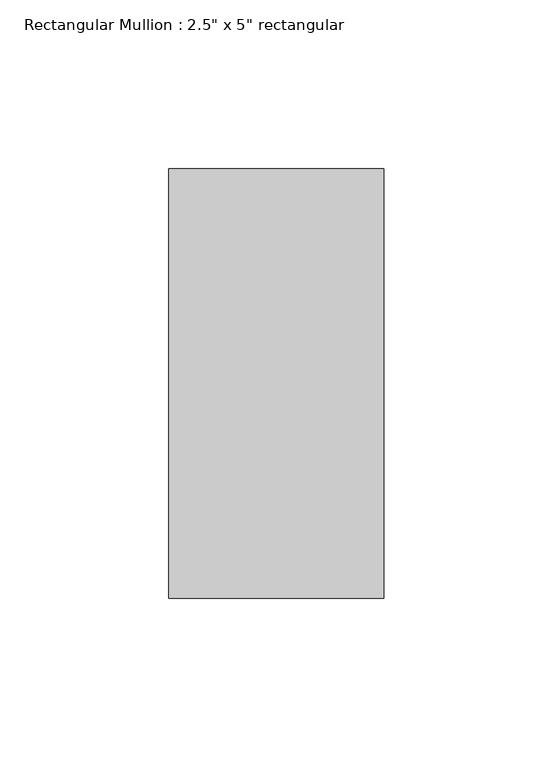
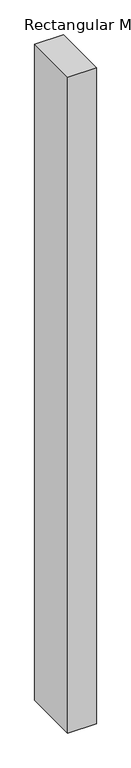
"""IFC4 building model written with IfcOpenShell, lengths in millimetres: member geometry."""

from ifc_helpers import new_model, si_unit, frame, origin, place, context, project, spatial, polyline, outline, extrude, source, transform, mapped, element, save


def member_72dfeae6(model_context):
    return source(origin(), model_context, "Body", "SweptSolid", [
        extrude(outline(polyline([(31.75, 63.5), (31.75, -63.5), (-31.75, -63.5), (-31.75, 63.5), (31.75, 63.5)])), frame((0.0, 0.0, -1539.658794), z_axis=(0.0, 0.0, 1.0), x_axis=(1.0, 0.0, 0.0)), (0.0, 0.0, 1.0), 1539.658794),
    ])


if __name__ == "__main__":
    model = new_model("IFC4")
    model_context = context("Model", 3, world=origin())
    ifc_project = project(units=[si_unit("LENGTHUNIT", "METRE", prefix="MILLI")], contexts=[model_context])
    site = spatial("IfcSite", under=ifc_project)
    building = spatial("IfcBuilding", under=site)
    placement = place(None, origin())
    member_shape = member_72dfeae6(model_context)
    element("IfcMember", 1, ObjectType="Rectangular Mullion : 2.5\" x 5\" rectangular", at=placement, inside=building, context=model_context, shape_type="MappedRepresentation", body=[
        mapped(member_shape, transform((0.0, 0.0, 0.0), x_axis=(1.0, 0.0, 0.0), y_axis=(0.0, 1.0, 0.0), z_axis=(0.0, 0.0, 1.0))),
    ])
    save(model, "model.ifc")

# Revit data of these elements
# Type "Rectangular Mullion : 2.5\" x 5\" rectangular"
#   built-in parameter 1007304 = 0.416667 (stored number, unit not read)
#   built-in parameter 1007301 = 0.104167 (stored number, unit not read)
#   built-in parameter 1007300 = 0.104167 (stored number, unit not read)
# Element 1 (IfcMember, "Rectangular Mullion : 2.5\" x 5\" rectangular")
#   Materials on its faces: "Aluminum"
# Materials
#   "Aluminum": class "Metal", colour RGB 247 247 247, transparency 0, Description = "Aluminum 6061", Cost = 0
